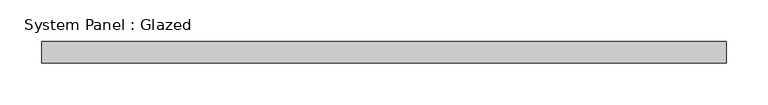
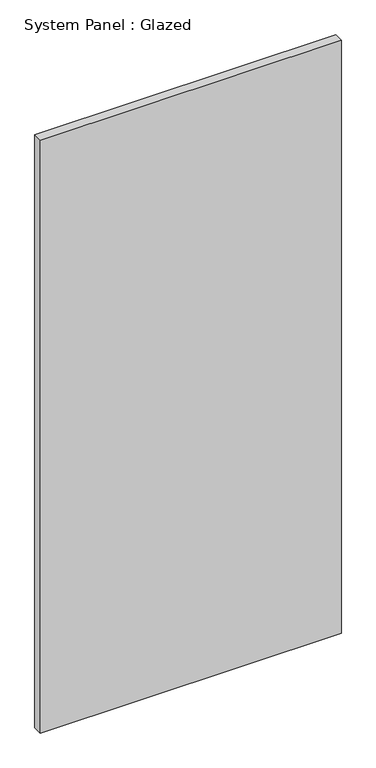
"""IFC4 building model written with IfcOpenShell, lengths in millimetres: plate geometry, System Panel : Glazed."""

from ifc_helpers import new_model, si_unit, origin, origin_with_axes, place, context, project, spatial, polyline, outline, extrude, source, transform, mapped, element, save


def system_panel_glazed_a7ecbca6(model_context):
    return source(origin(), model_context, "Body", "SweptSolid", [
        extrude(outline(polyline([(408.825192, -44.45), (-408.825192, -44.45), (-408.825192, -19.05), (408.825192, -19.05), (408.825192, -44.45)])), origin_with_axes(), (0.0, 0.0, 1.0), 1701.8),
    ])


if __name__ == "__main__":
    model = new_model("IFC4")
    model_context = context("Model", 3, world=origin())
    ifc_project = project(units=[si_unit("LENGTHUNIT", "METRE", prefix="MILLI")], contexts=[model_context])
    site = spatial("IfcSite", under=ifc_project)
    building = spatial("IfcBuilding", under=site)
    placement = place(None, origin())
    system_panel_glazed_shape = system_panel_glazed_a7ecbca6(model_context)
    element("IfcPlate", 1, ObjectType="System Panel : Glazed", at=placement, inside=building, context=model_context, shape_type="MappedRepresentation", body=[
        mapped(system_panel_glazed_shape, transform((0.0, 0.0, 0.0), x_axis=(1.0, 0.0, 0.0), y_axis=(0.0, 1.0, 0.0), z_axis=(0.0, 0.0, 1.0))),
    ])
    save(model, "model.ifc")

# Revit data of these elements
# Type "System Panel : Glazed"
#   Construction Type Id = "GSP4R"
#   Analytic Construction = "1/8 in Pilkington single glazing"
#   Visual Light Transmittance = 0.9
#   Solar Heat Gain Coefficient = 0.86
#   Heat Transfer Coefficient (U) = 1.18115 BTU/(h·ft²·°F)
#   Define Thermal Properties by = 1
# Element 1 (IfcPlate, "System Panel : Glazed")
#   Materials on its faces: "Glass"
# Materials
#   "Glass": class "Glass", colour RGB 0 128 192, transparency 0.75, Description = "Soda Lime Glass", Cost = 0
